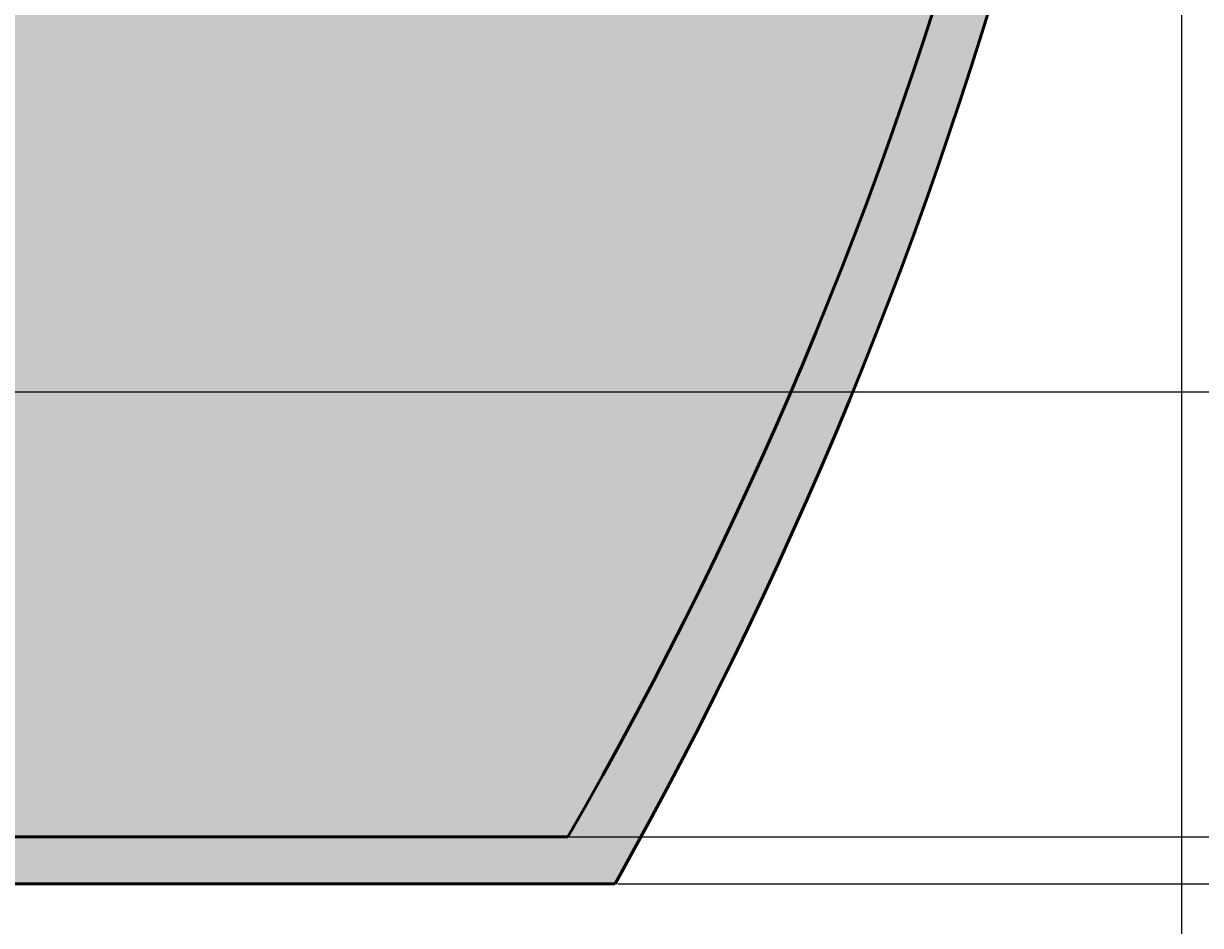
# Model space of a CAD drawing. Units: inches. Extents: x -12 to 334, y -10 to 186.
# Tile 70 of 77: x 257 to 282, y 45 to 64. Entities that reach past the tile are written whole.
import ezdxf
from ezdxf import colors
from ezdxf.entities.mleader import LeaderData, LeaderLine
from ezdxf.math import Vec2, Vec3

# ---------------------------------------------------------------- set-up
doc = ezdxf.new("R2010")
doc.units = ezdxf.units.IN
doc.header["$MEASUREMENT"] = 0
for name, color, linetype, lineweight in [('M-ANNO-TEXT', 3, 'Continuous', 25), ('M-DIMS', 2, 'Continuous', 18), ('M-EQPM', 7, 'Continuous', 50), ('M-EQPM-PATT', 8, 'Continuous', 18)]:
    doc.layers.add(name, color=color, linetype=linetype, lineweight=lineweight)
doc.styles.get("Standard").update_dxf_attribs({"font": 'arial.ttf'})
doc.dimstyles.get("Standard").update_dxf_attribs({"dimtxt": 0.18, "dimasz": 0.18, "dimexe": 0.18, "dimexo": 0.0625, "dimgap": 0.09, "dimtad": 0, "dimtih": 1, "dimtoh": 1, "dimdec": 4, "dimzin": 0, "dimdsep": 46, "dimtxsty": 'Standard', "dimcen": 0.09, "dimadec": 0, "dimazin": 0, "dimtfac": 1, "dimtdec": 4, "dimtofl": 0, "dimtmove": 0, "dimatfit": 3, "dimfxl": 1, "dimtolj": 1, "dimtzin": 0, "dimarcsym": 0})

# ---------------------------------------------------------------- blocks, each defined once
blk = doc.blocks.new('*D1')
at = {"layer": 'Defpoints', "color": 0, "transparency": 16777216}
for p in [(281.426, 91.899), (3.376, 80.692), (281.426, 14.304)]:
    blk.add_point(p, dxfattribs=at)
at = {"layer": 'M-DIMS', "color": 0, "lineweight": -2, "transparency": 16777216}
for p, q in [((281.426, 91.836), (281.426, 14.124)), ((3.376, 80.629), (3.376, 14.124)), ((3.556, 14.304), (141.935, 14.304)), ((281.246, 14.304), (142.867, 14.304))]:
    blk.add_line(p, q, dxfattribs=at)
at = {"layer": 'M-DIMS', "color": 0, "transparency": 16777216}
for points in [[(3.556, 14.334), (3.556, 14.274), (3.376, 14.304)], [(281.246, 14.334), (281.246, 14.274), (281.426, 14.304)]]:
    blk.add_solid(points, dxfattribs=at)
at = {"layer": 'M-DIMS', "color": 0, "transparency": 16777216, "insert": (142.401, 14.304), "char_height": 0.18, "attachment_point": 5}
blk.add_mtext('\\A1;278.05', dxfattribs=at)
blk = doc.blocks.new('*D17')
at = {"layer": 'Defpoints', "color": 0, "transparency": 16777216}
for p in [(106.177, 102.896), (105.892, 56.321), (295.976, 56.321)]:
    blk.add_point(p, dxfattribs=at)
at = {"layer": 'M-DIMS', "color": 0, "lineweight": -2, "transparency": 16777216}
for p, q in [((106.24, 102.896), (296.156, 102.896)), ((295.976, 102.716), (295.976, 79.79)), ((295.976, 56.501), (295.976, 79.426)), ((105.954, 56.321), (296.156, 56.321))]:
    blk.add_line(p, q, dxfattribs=at)
at = {"layer": 'M-DIMS', "color": 0, "transparency": 16777216}
for points in [[(295.946, 102.716), (296.006, 102.716), (295.976, 102.896)], [(295.946, 56.501), (296.006, 56.501), (295.976, 56.321)]]:
    blk.add_solid(points, dxfattribs=at)
at = {"layer": 'M-DIMS', "color": 0, "transparency": 16777216, "insert": (295.976, 79.608), "char_height": 0.18, "attachment_point": 5}
blk.add_mtext('\\A1;46.575', dxfattribs=at)
blk = doc.blocks.new('*D24')
at = {"layer": 'Defpoints', "color": 0, "transparency": 16777216}
for p in [(269.381, 137.943), (269.381, 45.854), (295.976, 45.854)]:
    blk.add_point(p, dxfattribs=at)
at = {"layer": 'M-DIMS', "color": 0, "lineweight": -2, "transparency": 16777216}
for p, q in [((269.443, 137.943), (296.156, 137.943)), ((295.976, 137.763), (295.976, 92.081)), ((295.976, 46.034), (295.976, 91.717)), ((269.443, 45.854), (296.156, 45.854))]:
    blk.add_line(p, q, dxfattribs=at)
at = {"layer": 'M-DIMS', "color": 0, "transparency": 16777216}
for points in [[(295.946, 137.763), (296.006, 137.763), (295.976, 137.943)], [(295.946, 46.034), (296.006, 46.034), (295.976, 45.854)]]:
    blk.add_solid(points, dxfattribs=at)
at = {"layer": 'M-DIMS', "color": 0, "transparency": 16777216, "insert": (295.976, 91.899), "char_height": 0.18, "attachment_point": 5}
blk.add_mtext('\\A1;92.09', dxfattribs=at)
blk = doc.blocks.new('*D38')
at = {"layer": 'Defpoints', "color": 0, "transparency": 16777216}
for p in [(247.935, 82.697), (247.935, 46.854), (295.976, 46.854)]:
    blk.add_point(p, dxfattribs=at)
at = {"layer": 'M-DIMS', "color": 0, "lineweight": -2, "transparency": 16777216}
for p, q in [((247.998, 82.697), (296.156, 82.697)), ((295.976, 82.517), (295.976, 64.957)), ((295.976, 47.034), (295.976, 64.594)), ((247.998, 46.854), (296.156, 46.854))]:
    blk.add_line(p, q, dxfattribs=at)
at = {"layer": 'M-DIMS', "color": 0, "transparency": 16777216}
for points in [[(295.946, 82.517), (296.006, 82.517), (295.976, 82.697)], [(295.946, 47.034), (296.006, 47.034), (295.976, 46.854)]]:
    blk.add_solid(points, dxfattribs=at)
at = {"layer": 'M-DIMS', "color": 0, "transparency": 16777216, "insert": (295.976, 64.775), "char_height": 0.18, "attachment_point": 5}
blk.add_mtext('\\A1;35.84', dxfattribs=at)
blk = doc.blocks.new('*D39')
at = {"layer": 'Defpoints', "color": 0, "transparency": 16777216}
for p in [(279.726, 80.692), (-11.174, 45.854), (269.381, 45.854)]:
    blk.add_point(p, dxfattribs=at)
at = {"layer": 'M-DIMS', "color": 0, "lineweight": -2, "transparency": 16777216}
for p, q in [((279.664, 80.692), (-11.354, 80.692)), ((-11.174, 80.512), (-11.174, 63.455)), ((-11.174, 46.034), (-11.174, 63.091)), ((269.318, 45.854), (-11.354, 45.854))]:
    blk.add_line(p, q, dxfattribs=at)
at = {"layer": 'M-DIMS', "color": 0, "transparency": 16777216}
for points in [[(-11.204, 80.512), (-11.144, 80.512), (-11.174, 80.692)], [(-11.204, 46.034), (-11.144, 46.034), (-11.174, 45.854)]]:
    blk.add_solid(points, dxfattribs=at)
at = {"layer": 'M-DIMS', "color": 0, "transparency": 16777216, "insert": (-11.174, 63.273), "char_height": 0.18, "attachment_point": 5}
blk.add_mtext('\\A1;34.84', dxfattribs=at)
blk = doc.blocks.new('*D41')
at = {"layer": 'Defpoints', "color": 0, "transparency": 16777216}
for p in [(190.169, 91.899), (277.343, 68.515)]:
    blk.add_point(p, dxfattribs=at)
at = {"layer": 'M-DIMS', "color": 0, "lineweight": -2, "transparency": 16777216}
for p, q in [((190.079, 91.899), (190.259, 91.899)), ((190.169, 91.809), (190.169, 91.989)), ((329.648, 54.485), (277.517, 68.469)), ((329.828, 54.485), (329.648, 54.485))]:
    blk.add_line(p, q, dxfattribs=at)
at = {"layer": 'M-DIMS', "color": 0, "transparency": 16777216}
blk.add_solid([(277.525, 68.498), (277.509, 68.44), (277.343, 68.515)], dxfattribs=at)
at = {"layer": 'M-DIMS', "color": 0, "transparency": 16777216, "insert": (330.307, 54.485), "char_height": 0.18, "attachment_point": 5}
blk.add_mtext('\\A1;R90.26', dxfattribs=at)

msp = doc.modelspace()

# ---------------------------------------------------------------- hatches: boundary and pattern name
at = {"layer": 'M-EQPM-PATT'}
h = msp.add_hatch(color=256, dxfattribs=at)
h.set_gradient(color1=(99, 100, 102), color2=(99, 100, 102), tint=1)
h.paths.add_polyline_path([(126.9567, 136.8871), (179.7818, 136.8871), (180.0106, 137.8871), (126.3793, 137.8871), (106.1771, 102.8958), (86.8879, 102.8958), (86.8879, 109.0583), (84.7229, 109.0583), (84.7229, 100.8958), (106.1771, 100.8958)])
h.paths.add_polyline_path([(196.3421, 152.8345), (195.3421, 152.8345), (195.3421, 137.8871), (180.0106, 137.8871), (179.7818, 136.8871), (196.3421, 136.8871)])
h.paths.add_polyline_path([(215.0166, 152.8345), (214.0166, 152.8345), (214.0166, 136.9435), (268.3808, 136.9435, -0.2673785), (268.3808, 46.8541), (249.3759, 46.8541), (249.8485, 45.8541), (269.3808, 45.8541, 0.2615891), (269.3808, 137.9435), (215.0166, 137.9435)])
h = msp.add_hatch(color=256, dxfattribs=at)
h.set_gradient(color1=(94, 103, 175), color2=(94, 103, 175), tint=1)
h.paths.add_polyline_path([(129.093, 89.8963), (86.8879, 89.8963), (86.8879, 69.6117), (129.093, 69.6117)], flags=17)
h.paths.add_polyline_path([(170.9079, 89.8963), (130.8573, 89.8963), (130.8573, 69.6117), (170.9079, 69.6117)], flags=17)
h.paths.add_polyline_path([(216.4278, 89.8963), (172.6722, 89.8963), (172.6722, 69.6117), (216.4278, 69.6117)], flags=17)
h.paths.add_polyline_path([(245.9354, 82.6969), (247.9354, 82.6969), (247.9354, 46.8541), (268.3808, 46.8541, 0.0998398), (279.7263, 80.6915), (251.9801, 80.6915, 0.4142136), (231.7758, 100.8958), (84.7229, 100.8958), (84.7229, 109.0583), (83.7229, 109.0583), (83.7229, 95.8963), (129.093, 95.8963), (129.093, 98.1081), (130.8573, 98.1081), (130.8573, 95.8963), (170.9079, 95.8963), (170.9079, 98.1081), (172.6722, 98.1081), (172.6722, 95.8963), (216.4278, 95.8963), (216.4278, 98.1081), (218.1922, 98.1081), (218.1922, 95.8963), (226.6083, 95.8963, -1), (226.6083, 63.6117), (218.1922, 63.6117), (218.1922, 61.1045), (216.4278, 61.1045), (216.4278, 63.6117), (172.6722, 63.6117), (172.6722, 61.1045), (170.9079, 61.1045), (170.9079, 63.6117), (130.8573, 63.6117), (130.8573, 61.1045), (129.093, 61.1045), (129.093, 63.6117), (87.8879, 63.6117), (87.8879, 56.3205), (105.8919, 56.3205), (105.8919, 28.8541), (115.8919, 28.8541), (115.8919, 46.8541), (222.5761, 46.8541), (222.5761, 30.8541), (232.5761, 30.8541), (232.5761, 46.8541), (245.9354, 46.8541)])
h.paths.add_polyline_path([(86.8879, 89.8963), (75.9244, 89.8963), (75.9244, 69.6117), (86.8879, 69.6117)])
h.paths.add_polyline_path([(83.7229, 109.0583), (75.9244, 109.0583), (75.9244, 95.8963), (83.7229, 95.8963)])
h.paths.add_polyline_path([(226.6083, 89.8963), (218.1922, 89.8963), (218.1922, 69.6117), (226.6083, 69.6117, 1)], flags=17)
h = msp.add_hatch(color=256, dxfattribs=at)
h.set_gradient(color1=(0, 0, 255), color2=(0, 0, 255), tint=1)
h.paths.add_polyline_path([(84.7229, 100.8958), (84.7229, 109.0583), (83.7229, 109.0583), (83.7229, 95.8963), (129.093, 95.8963), (129.093, 98.1081), (130.8573, 98.1081), (130.8573, 95.8963), (170.9079, 95.8963), (170.9079, 98.1081), (172.6722, 98.1081), (172.6722, 95.8963), (216.4278, 95.8963), (216.4278, 98.1081), (218.1922, 98.1081), (218.1922, 95.8963), (226.6083, 95.8963, -1), (226.6083, 63.6117), (218.1922, 63.6117), (218.1922, 61.1045), (216.4278, 61.1045), (216.4278, 63.6117), (172.6722, 63.6117), (172.6722, 61.1045), (170.9079, 61.1045), (170.9079, 63.6117), (130.8573, 63.6117), (130.8573, 61.1045), (129.093, 61.1045), (129.093, 63.6117), (87.8879, 63.6117), (87.8879, 56.3205), (105.8919, 56.3205), (105.8919, 28.8541), (115.8919, 28.8541), (115.8919, 46.8541), (222.5761, 46.8541), (222.5761, 30.8541), (232.5761, 30.8541), (232.5761, 46.8541), (245.9354, 46.8541), (245.9354, 82.6969), (247.9354, 82.6969), (247.9354, 46.8541), (268.3808, 46.8541, 0.0998398), (279.7263, 80.6915), (251.9801, 80.6915, 0.4142136), (231.7758, 100.8958)])

# ---------------------------------------------------------------- linework, layer by layer
at = {"layer": 'M-EQPM'}
for p, q in [((268.3808, 46.8541), (232.5761, 46.8541)), ((269.3808, 45.8541), (233.5761, 45.8541)), ((269.3808, 45.8541), (269.3808, 45.8541))]:
    msp.add_line(p, q, dxfattribs=at)
for centre, radius, start, end in [((187.3936, 91.8988), 94.032, 330.681071, 29.318929), ((190.1689, 91.8988), 90.256, 330.061028, 29.938972)]:
    msp.add_arc(centre, radius, start, end, dxfattribs=at)

# ---------------------------------------------------------------- dimensions: what is measured, and where the dimension line sits
at = {"layer": 'M-DIMS'}
for base, p1, p2, override, picture, middle in [((295.9756, 45.8541), (269.3808, 137.9435), (269.3808, 45.8541), {"dimdec": 2, "dimlfac": 1, "dimrnd": 0, "dimzin": 0, "dimdsep": 46, "dimlunit": 2}, '*D24', (295.9756, 91.8988)), ((295.9756, 56.3205), (106.1771, 102.8958), (105.8919, 56.3205), {"dimdec": 3, "dimlfac": 1, "dimrnd": 0, "dimzin": 0, "dimdsep": 46, "dimlunit": 2}, '*D17', (295.9756, 79.6082)), ((295.9756, 46.8541), (247.9354, 82.6969), (247.9354, 46.8541), {"dimdec": 2, "dimlfac": 1, "dimrnd": 0, "dimzin": 0, "dimdsep": 46, "dimlunit": 2}, '*D38', (295.9756, 64.7755)), ((-11.1736, 45.8541), (279.7263, 80.6915), (269.3808, 45.8541), {"dimdec": 2, "dimlfac": 1, "dimrnd": 0, "dimzin": 0, "dimdsep": 46, "dimlunit": 2}, '*D39', (-11.1735, 63.2728))]:
    dim = msp.add_linear_dim(base=base, p1=p1, p2=p2, angle=90, dimstyle='Standard', override=override, dxfattribs=at)
    dim.commit()
    dim.dimension.update_dxf_attribs({"geometry": picture, "text_midpoint": middle})
dim = msp.add_linear_dim(base=(281.4256, 14.3041), p1=(3.3765, 80.6915), p2=(281.4256, 91.8988), dimstyle='Standard', override={"dimdec": 2, "dimlfac": 1, "dimrnd": 0, "dimzin": 0, "dimdsep": 46, "dimlunit": 2}, dxfattribs=at)
dim.commit()
dim.dimension.update_dxf_attribs({"geometry": '*D1', "text_midpoint": (142.401, 14.3041)})
dim = msp.add_radius_dim(center=(190.1689, 91.8988), mpoint=(277.3431, 68.5153), dimstyle='Standard', override={"dimdec": 2, "dimlfac": 1, "dimrnd": 0, "dimzin": 0, "dimdsep": 46, "dimlunit": 2}, dxfattribs=at)
dim.commit()
dim.dimension.update_dxf_attribs({"geometry": '*D41', "text_midpoint": (330.3074, 54.4851), "dimtype": 164})

# ---------------------------------------------------------------- leaders
at = {"layer": 'M-ANNO-TEXT'}
ml = msp.add_multileader_mtext('Standard', dxfattribs=at)
ml.set_content('^I^IWeir', color=256)
ml.set_leader_properties()
ml.build(insert=Vec2(0, 0))
ml.multileader.update_dxf_attribs({"dogleg_length": 0.36, "arrow_head_size": 0.7})
ctx = ml.context
ctx.base_point, ctx.arrow_head_size, ctx.landing_gap_size, ctx.plane_origin = Vec3(257.1525, 34.1955), 0.7, 0.09, Vec3(247.9354, 49.9015)
notes = []
notes.append((ctx, [(0, (1, 1, 0), (255.3593, 34.1955), (1, 0), 1.7932, [(0, [(247.9354, 49.9015)], 0, [])])]))
ctx.mtext.insert, ctx.mtext.flow_direction = Vec3(257.2425, 36.2283), 5
for ctx, leaders in notes:
    for number, flags, end, landing, length, lines in leaders:
        leader = LeaderData()
        leader.index, (leader.has_last_leader_line, leader.has_dogleg_vector, leader.attachment_direction) = number, flags
        leader.last_leader_point, leader.dogleg_vector, leader.dogleg_length = Vec3(end), Vec3(landing), length
        for number, points, colour, breaks in lines:
            line = LeaderLine()
            line.index, line.vertices, line.color, line.breaks = number, Vec3.list(points), colors.encode_raw_color(colour), breaks
            leader.lines.append(line)
        ctx.leaders.append(leader)

doc.saveas('drawing.dxf')
